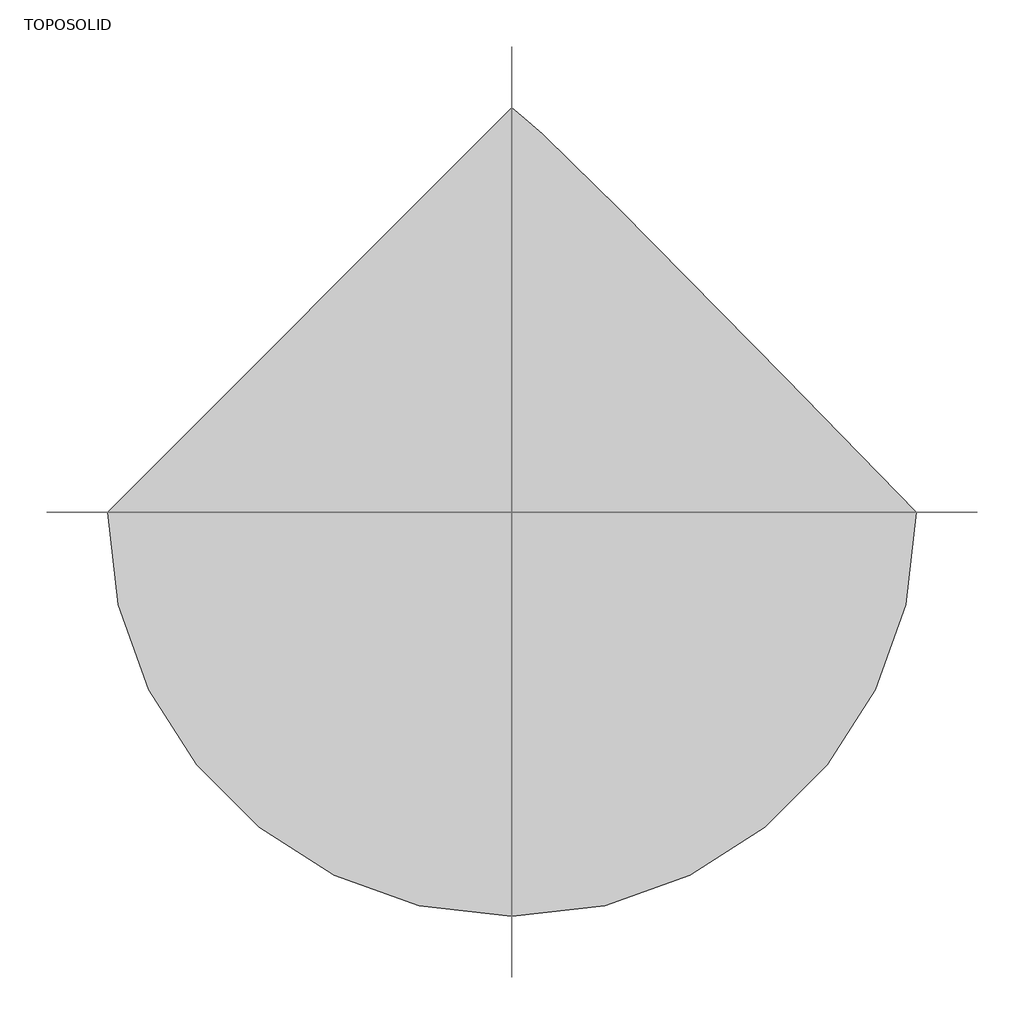
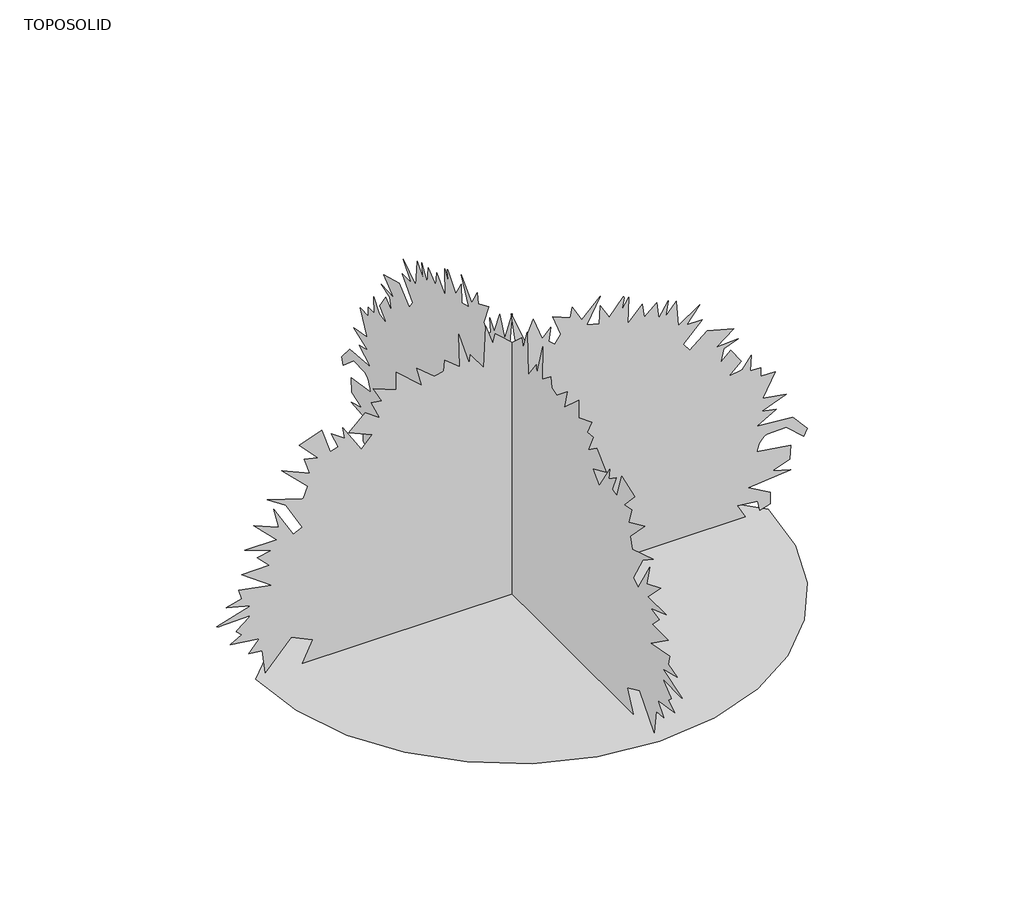
# One storey: 1 geographic element.
"""IFC4 building model written with IfcOpenShell, lengths in millimetres."""

from ifc_helpers import new_model, si_unit, origin, place, context, project, spatial, transform, mapped, element, save
from components import m_rpc_shrub_juniper_0_92_meters_8f64cf4e

model = new_model("IFC4")

# Units and contexts
model_context = context("Model", 3, world=origin())
ifc_project = project(units=[si_unit("LENGTHUNIT", "METRE", prefix="MILLI")], contexts=[model_context])

# Site, building, storey
site = spatial("IfcSite", under=ifc_project)
building = spatial("IfcBuilding", under=site)
storey = spatial("IfcBuildingStorey", under=building, Name="TOPOSOLID", Elevation=-254.0)

# Geographic element
placement = place(None, origin())
m_rpc_shrub_juniper_0_92_meters_shape = m_rpc_shrub_juniper_0_92_meters_8f64cf4e(model_context)
element("IfcGeographicElement", 1, ObjectType="M_RPC Shrub : Juniper - 0.92 Meters", at=placement, inside=storey, context=model_context, shape_type="MappedRepresentation", body=[
    mapped(m_rpc_shrub_juniper_0_92_meters_shape, transform((-1879.8317552, -5466.7477501, -254.0), x_axis=(1.0, 0.0, 0.0), y_axis=(0.0, 1.0, 0.0), z_axis=(0.0, 0.0, 1.0))),
])

save(model, "model.ifc")

# Revit data of these elements
# Type "M_RPC Shrub : Juniper - 0.92 Meters"
#   Type Comments = "Juniper"
#   built-in parameter 1005198 = "{2, 15},{39, RPC-16-FU4H-UTPX-8HVP-A000-ST1L-LVER-AU},{1, 0},{1, 0},{2, 35},{1, 8},{5, Color},{1, 0},{1, 0},{3, 0.8},{3, 0.8},{3, 0.8},{1, 8},{7, BBoxMin},{1, 0},{1, 0},{1, 0},{1, 0},{1, 0},{1, 8},{7, BBoxMax},{1, 0},{1, 0},{1, 0},{1, 0},{1, 0},{2, 11},{9, RPCTypeId},{1, 0},{1, 0},{39, RPC-16-FU4H-UTPX-8HVP-A000-ST1L-LVER-AU},{1, 6},{14, RPCPlantHeight},{1, 0},{1, 0},{7, 3.01837},{2, 11},{7, keyword},{1, 0},{1, 0},{21, :Geometry:RPC:Juniper},{2, 11},{8, category},{1, 0},{1, 0},{17, :Shrubs & Grasses},{2, 11},{12, LocalizedUID},{1, 0},{1, 0},{7, Juniper},{2, 14},{6, Height},{1, 0},{1, 0},{7, 3.01837},{1, 2},{16, Cast Reflections},{1, 0},{1, 0},{1, 0},{1, 2},{12, Cast Shadows},{1, 0},{1, 0},{1, 1},{1, 2},{9, Lock View},{1, 0},{1, 0},{1, 0},{1, 4},{5, ViewC},{1, 0},{1, 0},{1, 0},{2, 11},{20, AdvancedUIDefinition},{1, 0},{1, 0},{0, },{2, 11},{10, AssetLibID},{1, 0},{1, 0},{36, 4D3F6E72-3F99-4203-98E9-AF80B3C7A7A4},{2, 11},{10, BaseSchema},{1, 0},{1, 0},{9, RPCSchema},{2, 11},{12, ExchangeGUID},{1, 0},{1, 0},{0, },{1, 2},{6, Hidden},{1, 0},{1, 0},{1, 0},{1, 4},{11, RPCCategory},{1, 0},{1, 0},{1, 0},{2, 11},{8, RPCImage},{1, 0},{1, 0},{0, },{1, 4},{13, SchemaVersion},{1, 0},{1, 0},{1, 4},{2, 11},{12, UIDefinition},{1, 0},{1, 0},{0, },{2, 11},{6, UIName},{1, 0},{1, 0},{39, RPC-16-FU4H-UTPX-8HVP-A000-ST1L-LVER-AU},{2, 11},{11, VersionGUID},{1, 0},{1, 0},{9, RPCSchema},{2, 11},{9, assettype},{1, 0},{1, 0},{11, RPCGeometry},{2, 11},{11, description},{1, 0},{1, 0},{0, },{2, 11},{9, localname},{1, 0},{1, 0},{3, RPC},{2, 11},{9, localtype},{1, 0},{1, 0},{3, RPC},{1, 4},{8, revision},{1, 0},{1, 0},{1, 1},{2, 11},{9, thumbnail},{1, 0},{1, 0},{0, },{1, 4},{7, version},{1, 0},{1, 0},{1, 1},{1, 2},{20, RPC_Cast Reflections},{1, 0},{1, 0},{1, 1},{1, 2},{16, RPC_Cast Shadows},{1, 0},{1, 0},{1, 1},{1, 2},{13, RPC_Lock View},{1, 0},{1, 0},{1, 0},{1, 4},{9, RPC_ViewC},{1, 0},{1, 0},{1, 0},{21, assetlibrary_base.fbx},{1, 5},"
#   built-in parameter 1005195 = "RPC-16-FU4H-UTPX-8HVP-A000-ST1L-LVER-AU"
#   Height = 920 mm
#   Description = (empty or 0)
#   Default Elevation = 0
# Element 1 (IfcGeographicElement, "M_RPC Shrub : Juniper - 0.92 Meters")
#   Phase Created = New Construction
